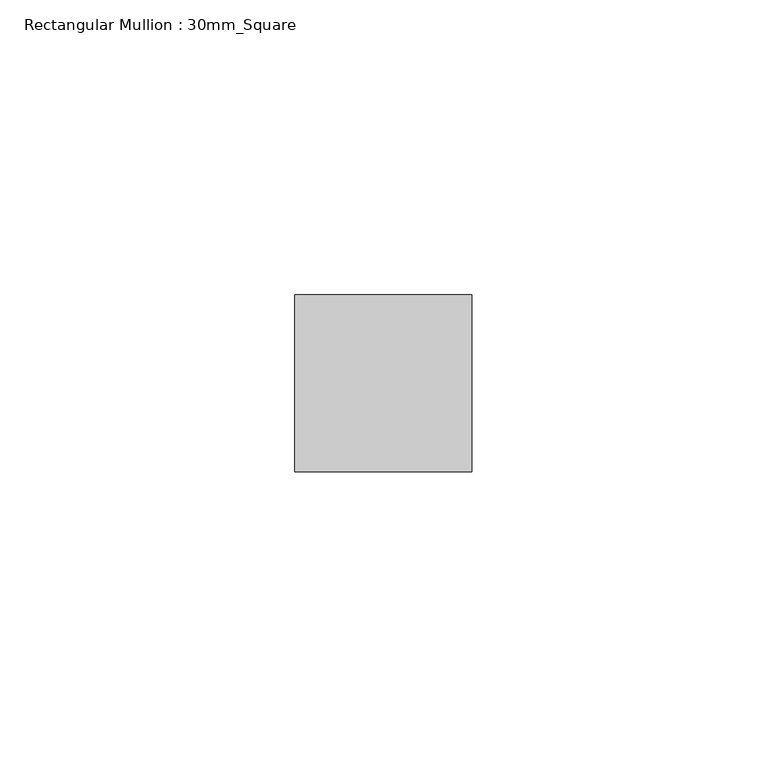
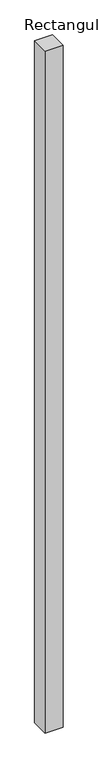
"""IFC4 building model written with IfcOpenShell, lengths in millimetres: member geometry, Rectangular Mullion : 30mm_Square."""

from ifc_helpers import new_model, si_unit, frame, origin, place, context, project, spatial, polyline, outline, extrude, source, transform, mapped, element, save


def rectangular_mullion_30mm_square_bfb5791d(model_context):
    return source(origin(), model_context, "Body", "SweptSolid", [
        extrude(outline(polyline([(0.0, 15.0), (0.0, -15.0), (-30.0, -15.0), (-30.0, 15.0), (0.0, 15.0)])), frame((0.0, 0.0, -1206.1333331), z_axis=(0.0, 0.0, 1.0), x_axis=(1.0, 0.0, 0.0)), (0.0, 0.0, 1.0), 1206.1333331),
    ])


if __name__ == "__main__":
    model = new_model("IFC4")
    model_context = context("Model", 3, world=origin())
    ifc_project = project(units=[si_unit("LENGTHUNIT", "METRE", prefix="MILLI")], contexts=[model_context])
    site = spatial("IfcSite", under=ifc_project)
    building = spatial("IfcBuilding", under=site)
    placement = place(None, origin())
    rectangular_mullion_30mm_square_shape = rectangular_mullion_30mm_square_bfb5791d(model_context)
    element("IfcMember", 1, ObjectType="Rectangular Mullion : 30mm_Square", at=placement, inside=building, context=model_context, shape_type="MappedRepresentation", body=[
        mapped(rectangular_mullion_30mm_square_shape, transform((0.0, 0.0, 0.0), x_axis=(1.0, 0.0, 0.0), y_axis=(0.0, 1.0, 0.0), z_axis=(0.0, 0.0, 1.0))),
    ])
    save(model, "model.ifc")

# Revit data of these elements
# Type "Rectangular Mullion : 30mm_Square"
#   Keynote = "H11"
#   built-in parameter 1007304 = 0.0984252 (stored number, unit not read)
#   built-in parameter 1007301 = 0.0492126 (stored number, unit not read)
#   built-in parameter 1007300 = 0.0492126 (stored number, unit not read)
# Element 1 (IfcMember, "Rectangular Mullion : 30mm_Square")
#   Materials on its faces: "Aluminium"
# Materials
#   "Aluminium": class "Metal", colour RGB 247 247 247, transparency 0, Description = "Aluminium 6061", Cost = 0
